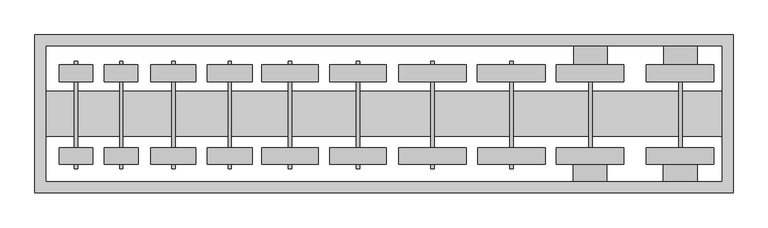
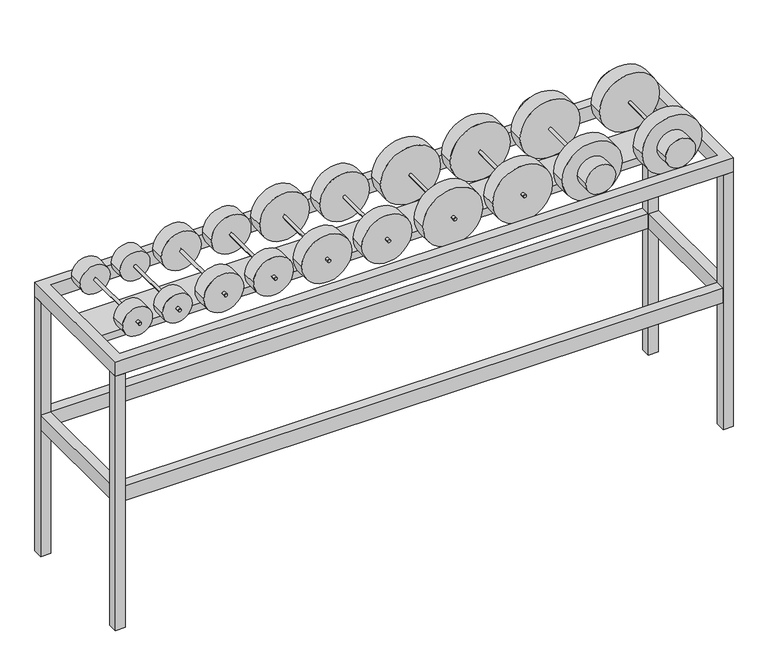
"""IFC4 building model written with IfcOpenShell, lengths in millimetres: proxy geometry."""

from ifc_helpers import new_model, si_unit, point, frame, frame_2d, origin, origin_with_axes, place, context, project, spatial, polyline, circle_curve, trimmed, segment, composite_curve, outline, extrude, source, transform, mapped, element, save


def specialty_equipment_60971a7b(model_context):
    return source(origin(), model_context, "Body", "SweptSolid", [
        extrude(outline(polyline([(-1032.0763254, -159.6107484), (-1032.0763254, 551.5892516), (2117.5236746, 551.5892516), (2117.5236746, -159.6107484), (-1032.0763254, -159.6107484)]), holes=[polyline([(-981.2763254, -108.8107484), (2066.7236746, -108.8107484), (2066.7236746, 500.7892516), (-981.2763254, 500.7892516), (-981.2763254, -108.8107484)])]), origin_with_axes(), (0.0, 0.0, 1.0), 76.2),
        extrude(outline(polyline([(-981.2763254, 500.7892516), (-1032.0763254, 500.7892516), (-1032.0763254, 551.5892516), (-981.2763254, 551.5892516), (-981.2763254, 500.7892516)])), frame((0.0, 0.0, -1371.6), z_axis=(0.0, 0.0, 1.0), x_axis=(1.0, 0.0, 0.0)), (0.0, 0.0, 1.0), 1371.6),
        extrude(outline(polyline([(-981.2763254, -159.6107484), (-1032.0763254, -159.6107484), (-1032.0763254, -108.8107484), (-981.2763254, -108.8107484), (-981.2763254, -159.6107484)])), frame((0.0, 0.0, -1371.6), z_axis=(0.0, 0.0, 1.0), x_axis=(1.0, 0.0, 0.0)), (0.0, 0.0, 1.0), 1371.6),
        extrude(outline(polyline([(2066.7236746, -159.6107484), (2066.7236746, -108.8107484), (2117.5236746, -108.8107484), (2117.5236746, -159.6107484), (2066.7236746, -159.6107484)])), frame((0.0, 0.0, -1371.6), z_axis=(0.0, 0.0, 1.0), x_axis=(1.0, 0.0, 0.0)), (0.0, 0.0, 1.0), 1371.6),
        extrude(outline(polyline([(2066.7236746, 500.7892516), (2066.7236746, 551.5892516), (2117.5236746, 551.5892516), (2117.5236746, 500.7892516), (2066.7236746, 500.7892516)])), frame((0.0, 0.0, -1371.6), z_axis=(0.0, 0.0, 1.0), x_axis=(1.0, 0.0, 0.0)), (0.0, 0.0, 1.0), 1371.6),
        extrude(outline(polyline([(-1032.0763254, -159.6107484), (-1032.0763254, 551.5892516), (2117.5236746, 551.5892516), (2117.5236746, -159.6107484), (-1032.0763254, -159.6107484)]), holes=[polyline([(-981.2763254, -108.8107484), (2066.7236746, -108.8107484), (2066.7236746, 500.7892516), (-981.2763254, 500.7892516), (-981.2763254, -108.8107484)])]), frame((0.0, 0.0, -685.8), z_axis=(0.0, 0.0, 1.0), x_axis=(1.0, 0.0, 0.0)), (0.0, 0.0, 1.0), 76.2),
        extrude(outline(composite_curve([segment(trimmed(circle_curve(frame_2d((154.4606082, -846.3325506)), 76.2), [point((154.4606082, -922.5325506))], [point((154.4606082, -770.1325506))], False, "CARTESIAN"), True, "CONTINUOUS"), segment(trimmed(circle_curve(frame_2d((154.4606082, -846.3325506)), 76.2), [point((154.4606082, -770.1325506))], [point((154.4606082, -922.5325506))], False, "CARTESIAN"), True, "CONTINUOUS")], self_intersect=False)), frame((0.0, -32.5823092, 0.0), z_axis=(0.0, 1.0, 0.0), x_axis=(0.0, 0.0, 1.0)), (0.0, 0.0, 1.0), 76.2),
        extrude(outline(polyline([(-981.2763254, 94.3892516), (-981.2763254, 297.5892516), (2066.7236746, 297.5892516), (2066.7236746, 94.3892516), (-981.2763254, 94.3892516)])), origin_with_axes(), (0.0, 0.0, 1.0), 38.1),
        extrude(outline(composite_curve([segment(trimmed(circle_curve(frame_2d((154.4606082, -846.6284427)), 76.2), [point((154.4606082, -922.8284427))], [point((154.4606082, -770.4284427))], False, "CARTESIAN"), True, "CONTINUOUS"), segment(trimmed(circle_curve(frame_2d((154.4606082, -846.6284427)), 76.2), [point((154.4606082, -770.4284427))], [point((154.4606082, -922.8284427))], False, "CARTESIAN"), True, "CONTINUOUS")], self_intersect=False)), frame((0.0, 341.3226899, 0.0), z_axis=(0.0, 1.0, 0.0), x_axis=(0.0, 0.0, 1.0)), (0.0, 0.0, 1.0), 76.2),
        extrude(outline(composite_curve([segment(trimmed(circle_curve(frame_2d((154.4606082, -845.747476)), 7.8489452), [point((154.4606082, -837.8985309))], [point((154.4606082, -853.5964212))], False, "CARTESIAN"), True, "CONTINUOUS"), segment(trimmed(circle_curve(frame_2d((154.4606082, -845.747476)), 7.8489452), [point((154.4606082, -853.5964212))], [point((154.4606082, -837.8985309))], False, "CARTESIAN"), True, "CONTINUOUS")], self_intersect=False)), frame((0.0, -53.073715, 0.0), z_axis=(0.0, 1.0, 0.0), x_axis=(0.0, 0.0, 1.0)), (0.0, 0.0, 1.0), 485.4827264),
        extrude(outline(composite_curve([segment(trimmed(circle_curve(frame_2d((154.4606082, -643.1325506)), 76.2), [point((154.4606082, -719.3325506))], [point((154.4606082, -566.9325506))], False, "CARTESIAN"), True, "CONTINUOUS"), segment(trimmed(circle_curve(frame_2d((154.4606082, -643.1325506)), 76.2), [point((154.4606082, -566.9325506))], [point((154.4606082, -719.3325506))], False, "CARTESIAN"), True, "CONTINUOUS")], self_intersect=False)), frame((0.0, -32.5823092, 0.0), z_axis=(0.0, 1.0, 0.0), x_axis=(0.0, 0.0, 1.0)), (0.0, 0.0, 1.0), 76.2),
        extrude(outline(composite_curve([segment(trimmed(circle_curve(frame_2d((154.4606082, -643.4284427)), 76.2), [point((154.4606082, -719.6284427))], [point((154.4606082, -567.2284427))], False, "CARTESIAN"), True, "CONTINUOUS"), segment(trimmed(circle_curve(frame_2d((154.4606082, -643.4284427)), 76.2), [point((154.4606082, -567.2284427))], [point((154.4606082, -719.6284427))], False, "CARTESIAN"), True, "CONTINUOUS")], self_intersect=False)), frame((0.0, 341.3226899, 0.0), z_axis=(0.0, 1.0, 0.0), x_axis=(0.0, 0.0, 1.0)), (0.0, 0.0, 1.0), 76.2),
        extrude(outline(composite_curve([segment(trimmed(circle_curve(frame_2d((154.4606082, -642.547476)), 7.8489452), [point((154.4606082, -634.6985309))], [point((154.4606082, -650.3964212))], False, "CARTESIAN"), True, "CONTINUOUS"), segment(trimmed(circle_curve(frame_2d((154.4606082, -642.547476)), 7.8489452), [point((154.4606082, -650.3964212))], [point((154.4606082, -634.6985309))], False, "CARTESIAN"), True, "CONTINUOUS")], self_intersect=False)), frame((0.0, -53.073715, 0.0), z_axis=(0.0, 1.0, 0.0), x_axis=(0.0, 0.0, 1.0)), (0.0, 0.0, 1.0), 485.4827264),
        extrude(outline(composite_curve([segment(trimmed(circle_curve(frame_2d((154.4606082, 1116.9227651)), 152.4), [point((154.4606082, 1269.3227651))], [point((154.4606082, 964.5227651))], False, "CARTESIAN"), True, "CONTINUOUS"), segment(trimmed(circle_curve(frame_2d((154.4606082, 1116.9227651)), 152.4), [point((154.4606082, 964.5227651))], [point((154.4606082, 1269.3227651))], False, "CARTESIAN"), True, "CONTINUOUS")], self_intersect=False)), frame((0.0, -32.5823092, 0.0), z_axis=(0.0, 1.0, 0.0), x_axis=(0.0, 0.0, 1.0)), (0.0, 0.0, 1.0), 76.2),
        extrude(outline(composite_curve([segment(trimmed(circle_curve(frame_2d((154.4606082, 1116.9227651)), 7.8489452), [point((154.4606082, 1124.7717102))], [point((154.4606082, 1109.0738199))], False, "CARTESIAN"), True, "CONTINUOUS"), segment(trimmed(circle_curve(frame_2d((154.4606082, 1116.9227651)), 7.8489452), [point((154.4606082, 1109.0738199))], [point((154.4606082, 1124.7717102))], False, "CARTESIAN"), True, "CONTINUOUS")], self_intersect=False)), frame((0.0, -53.073715, 0.0), z_axis=(0.0, 1.0, 0.0), x_axis=(0.0, 0.0, 1.0)), (0.0, 0.0, 1.0), 485.4827264),
        extrude(outline(composite_curve([segment(trimmed(circle_curve(frame_2d((154.4606082, 1116.7428206)), 152.4), [point((154.4606082, 1269.1428206))], [point((154.4606082, 964.3428206))], False, "CARTESIAN"), True, "CONTINUOUS"), segment(trimmed(circle_curve(frame_2d((154.4606082, 1116.7428206)), 152.4), [point((154.4606082, 964.3428206))], [point((154.4606082, 1269.1428206))], False, "CARTESIAN"), True, "CONTINUOUS")], self_intersect=False)), frame((0.0, 341.3226899, 0.0), z_axis=(0.0, 1.0, 0.0), x_axis=(0.0, 0.0, 1.0)), (0.0, 0.0, 1.0), 76.2),
        extrude(outline(composite_curve([segment(trimmed(circle_curve(frame_2d((154.4606082, 761.3227651)), 152.4), [point((154.4606082, 913.7227651))], [point((154.4606082, 608.9227651))], False, "CARTESIAN"), True, "CONTINUOUS"), segment(trimmed(circle_curve(frame_2d((154.4606082, 761.3227651)), 152.4), [point((154.4606082, 608.9227651))], [point((154.4606082, 913.7227651))], False, "CARTESIAN"), True, "CONTINUOUS")], self_intersect=False)), frame((0.0, -32.5823092, 0.0), z_axis=(0.0, 1.0, 0.0), x_axis=(0.0, 0.0, 1.0)), (0.0, 0.0, 1.0), 76.2),
        extrude(outline(composite_curve([segment(trimmed(circle_curve(frame_2d((154.4606082, 761.3227651)), 7.8489452), [point((154.4606082, 769.1717102))], [point((154.4606082, 753.4738199))], False, "CARTESIAN"), True, "CONTINUOUS"), segment(trimmed(circle_curve(frame_2d((154.4606082, 761.3227651)), 7.8489452), [point((154.4606082, 753.4738199))], [point((154.4606082, 769.1717102))], False, "CARTESIAN"), True, "CONTINUOUS")], self_intersect=False)), frame((0.0, -53.073715, 0.0), z_axis=(0.0, 1.0, 0.0), x_axis=(0.0, 0.0, 1.0)), (0.0, 0.0, 1.0), 485.4827264),
        extrude(outline(composite_curve([segment(trimmed(circle_curve(frame_2d((154.4606082, 761.1428206)), 152.4), [point((154.4606082, 913.5428206))], [point((154.4606082, 608.7428206))], False, "CARTESIAN"), True, "CONTINUOUS"), segment(trimmed(circle_curve(frame_2d((154.4606082, 761.1428206)), 152.4), [point((154.4606082, 608.7428206))], [point((154.4606082, 913.5428206))], False, "CARTESIAN"), True, "CONTINUOUS")], self_intersect=False)), frame((0.0, 341.3226899, 0.0), z_axis=(0.0, 1.0, 0.0), x_axis=(0.0, 0.0, 1.0)), (0.0, 0.0, 1.0), 76.2),
        extrude(outline(composite_curve([segment(trimmed(circle_curve(frame_2d((154.4606082, -407.0772349)), 101.6), [point((154.4606082, -305.4772349))], [point((154.4606082, -508.6772349))], False, "CARTESIAN"), True, "CONTINUOUS"), segment(trimmed(circle_curve(frame_2d((154.4606082, -407.0772349)), 101.6), [point((154.4606082, -508.6772349))], [point((154.4606082, -305.4772349))], False, "CARTESIAN"), True, "CONTINUOUS")], self_intersect=False)), frame((0.0, -32.5823092, 0.0), z_axis=(0.0, 1.0, 0.0), x_axis=(0.0, 0.0, 1.0)), (0.0, 0.0, 1.0), 76.2),
        extrude(outline(composite_curve([segment(trimmed(circle_curve(frame_2d((154.4606082, -407.0772349)), 7.8489452), [point((154.4606082, -399.2282898))], [point((154.4606082, -414.9261801))], False, "CARTESIAN"), True, "CONTINUOUS"), segment(trimmed(circle_curve(frame_2d((154.4606082, -407.0772349)), 7.8489452), [point((154.4606082, -414.9261801))], [point((154.4606082, -399.2282898))], False, "CARTESIAN"), True, "CONTINUOUS")], self_intersect=False)), frame((0.0, -53.073715, 0.0), z_axis=(0.0, 1.0, 0.0), x_axis=(0.0, 0.0, 1.0)), (0.0, 0.0, 1.0), 485.4827264),
        extrude(outline(composite_curve([segment(trimmed(circle_curve(frame_2d((154.4606082, -407.2571794)), 101.6), [point((154.4606082, -305.6571794))], [point((154.4606082, -508.8571794))], False, "CARTESIAN"), True, "CONTINUOUS"), segment(trimmed(circle_curve(frame_2d((154.4606082, -407.2571794)), 101.6), [point((154.4606082, -508.8571794))], [point((154.4606082, -305.6571794))], False, "CARTESIAN"), True, "CONTINUOUS")], self_intersect=False)), frame((0.0, 341.3226899, 0.0), z_axis=(0.0, 1.0, 0.0), x_axis=(0.0, 0.0, 1.0)), (0.0, 0.0, 1.0), 76.2),
        extrude(outline(composite_curve([segment(trimmed(circle_curve(frame_2d((154.4606082, -153.0772349)), 101.6), [point((154.4606082, -51.4772349))], [point((154.4606082, -254.6772349))], False, "CARTESIAN"), True, "CONTINUOUS"), segment(trimmed(circle_curve(frame_2d((154.4606082, -153.0772349)), 101.6), [point((154.4606082, -254.6772349))], [point((154.4606082, -51.4772349))], False, "CARTESIAN"), True, "CONTINUOUS")], self_intersect=False)), frame((0.0, -32.5823092, 0.0), z_axis=(0.0, 1.0, 0.0), x_axis=(0.0, 0.0, 1.0)), (0.0, 0.0, 1.0), 76.2),
        extrude(outline(composite_curve([segment(trimmed(circle_curve(frame_2d((154.4606082, -153.0772349)), 7.8489452), [point((154.4606082, -145.2282898))], [point((154.4606082, -160.9261801))], False, "CARTESIAN"), True, "CONTINUOUS"), segment(trimmed(circle_curve(frame_2d((154.4606082, -153.0772349)), 7.8489452), [point((154.4606082, -160.9261801))], [point((154.4606082, -145.2282898))], False, "CARTESIAN"), True, "CONTINUOUS")], self_intersect=False)), frame((0.0, -53.073715, 0.0), z_axis=(0.0, 1.0, 0.0), x_axis=(0.0, 0.0, 1.0)), (0.0, 0.0, 1.0), 485.4827264),
        extrude(outline(composite_curve([segment(trimmed(circle_curve(frame_2d((154.4606082, -153.2571794)), 101.6), [point((154.4606082, -51.6571794))], [point((154.4606082, -254.8571794))], False, "CARTESIAN"), True, "CONTINUOUS"), segment(trimmed(circle_curve(frame_2d((154.4606082, -153.2571794)), 101.6), [point((154.4606082, -254.8571794))], [point((154.4606082, -51.6571794))], False, "CARTESIAN"), True, "CONTINUOUS")], self_intersect=False)), frame((0.0, 341.3226899, 0.0), z_axis=(0.0, 1.0, 0.0), x_axis=(0.0, 0.0, 1.0)), (0.0, 0.0, 1.0), 76.2),
        extrude(outline(composite_curve([segment(trimmed(circle_curve(frame_2d((154.4606082, 119.2581533)), 127.0), [point((154.4606082, 246.2581533))], [point((154.4606082, -7.7418467))], False, "CARTESIAN"), True, "CONTINUOUS"), segment(trimmed(circle_curve(frame_2d((154.4606082, 119.2581533)), 127.0), [point((154.4606082, -7.7418467))], [point((154.4606082, 246.2581533))], False, "CARTESIAN"), True, "CONTINUOUS")], self_intersect=False)), frame((0.0, -32.5823092, 0.0), z_axis=(0.0, 1.0, 0.0), x_axis=(0.0, 0.0, 1.0)), (0.0, 0.0, 1.0), 76.2),
        extrude(outline(composite_curve([segment(trimmed(circle_curve(frame_2d((154.4606082, 119.2581533)), 7.8489452), [point((154.4606082, 127.1070985))], [point((154.4606082, 111.4092081))], False, "CARTESIAN"), True, "CONTINUOUS"), segment(trimmed(circle_curve(frame_2d((154.4606082, 119.2581533)), 7.8489452), [point((154.4606082, 111.4092081))], [point((154.4606082, 127.1070985))], False, "CARTESIAN"), True, "CONTINUOUS")], self_intersect=False)), frame((0.0, -53.073715, 0.0), z_axis=(0.0, 1.0, 0.0), x_axis=(0.0, 0.0, 1.0)), (0.0, 0.0, 1.0), 485.4827264),
        extrude(outline(composite_curve([segment(trimmed(circle_curve(frame_2d((154.4606082, 119.0782088)), 127.0), [point((154.4606082, 246.0782088))], [point((154.4606082, -7.9217912))], False, "CARTESIAN"), True, "CONTINUOUS"), segment(trimmed(circle_curve(frame_2d((154.4606082, 119.0782088)), 127.0), [point((154.4606082, -7.9217912))], [point((154.4606082, 246.0782088))], False, "CARTESIAN"), True, "CONTINUOUS")], self_intersect=False)), frame((0.0, 341.3226899, 0.0), z_axis=(0.0, 1.0, 0.0), x_axis=(0.0, 0.0, 1.0)), (0.0, 0.0, 1.0), 76.2),
        extrude(outline(composite_curve([segment(trimmed(circle_curve(frame_2d((154.4606082, 425.128062)), 127.0), [point((154.4606082, 552.128062))], [point((154.4606082, 298.128062))], False, "CARTESIAN"), True, "CONTINUOUS"), segment(trimmed(circle_curve(frame_2d((154.4606082, 425.128062)), 127.0), [point((154.4606082, 298.128062))], [point((154.4606082, 552.128062))], False, "CARTESIAN"), True, "CONTINUOUS")], self_intersect=False)), frame((0.0, -32.5823092, 0.0), z_axis=(0.0, 1.0, 0.0), x_axis=(0.0, 0.0, 1.0)), (0.0, 0.0, 1.0), 76.2),
        extrude(outline(composite_curve([segment(trimmed(circle_curve(frame_2d((154.4606082, 425.128062)), 7.8489452), [point((154.4606082, 432.9770072))], [point((154.4606082, 417.2791168))], False, "CARTESIAN"), True, "CONTINUOUS"), segment(trimmed(circle_curve(frame_2d((154.4606082, 425.128062)), 7.8489452), [point((154.4606082, 417.2791168))], [point((154.4606082, 432.9770072))], False, "CARTESIAN"), True, "CONTINUOUS")], self_intersect=False)), frame((0.0, -53.073715, 0.0), z_axis=(0.0, 1.0, 0.0), x_axis=(0.0, 0.0, 1.0)), (0.0, 0.0, 1.0), 485.4827264),
        extrude(outline(composite_curve([segment(trimmed(circle_curve(frame_2d((154.4606082, 424.9481175)), 127.0), [point((154.4606082, 551.9481175))], [point((154.4606082, 297.9481175))], False, "CARTESIAN"), True, "CONTINUOUS"), segment(trimmed(circle_curve(frame_2d((154.4606082, 424.9481175)), 127.0), [point((154.4606082, 297.9481175))], [point((154.4606082, 551.9481175))], False, "CARTESIAN"), True, "CONTINUOUS")], self_intersect=False)), frame((0.0, 341.3226899, 0.0), z_axis=(0.0, 1.0, 0.0), x_axis=(0.0, 0.0, 1.0)), (0.0, 0.0, 1.0), 76.2),
        extrude(outline(composite_curve([segment(trimmed(circle_curve(frame_2d((154.4606082, 1878.6053565)), 76.2), [point((154.4606082, 1802.4053565))], [point((154.4606082, 1954.8053565))], False, "CARTESIAN"), True, "CONTINUOUS"), segment(trimmed(circle_curve(frame_2d((154.4606082, 1878.6053565)), 76.2), [point((154.4606082, 1954.8053565))], [point((154.4606082, 1802.4053565))], False, "CARTESIAN"), True, "CONTINUOUS")], self_intersect=False)), frame((0.0, -108.7823092, 0.0), z_axis=(0.0, 1.0, 0.0), x_axis=(0.0, 0.0, 1.0)), (0.0, 0.0, 1.0), 76.2),
        extrude(outline(composite_curve([segment(trimmed(circle_curve(frame_2d((154.4606082, 1880.3392515)), 76.2), [point((154.4606082, 1804.1392515))], [point((154.4606082, 1956.5392515))], False, "CARTESIAN"), True, "CONTINUOUS"), segment(trimmed(circle_curve(frame_2d((154.4606082, 1880.3392515)), 76.2), [point((154.4606082, 1956.5392515))], [point((154.4606082, 1804.1392515))], False, "CARTESIAN"), True, "CONTINUOUS")], self_intersect=False)), frame((0.0, 417.5226899, 0.0), z_axis=(0.0, 1.0, 0.0), x_axis=(0.0, 0.0, 1.0)), (0.0, 0.0, 1.0), 83.2665617),
        extrude(outline(composite_curve([segment(trimmed(circle_curve(frame_2d((154.4606082, 1878.7428206)), 152.4), [point((154.4606082, 2031.1428206))], [point((154.4606082, 1726.3428206))], False, "CARTESIAN"), True, "CONTINUOUS"), segment(trimmed(circle_curve(frame_2d((154.4606082, 1878.7428206)), 152.4), [point((154.4606082, 1726.3428206))], [point((154.4606082, 2031.1428206))], False, "CARTESIAN"), True, "CONTINUOUS")], self_intersect=False)), frame((0.0, 341.3226899, 0.0), z_axis=(0.0, 1.0, 0.0), x_axis=(0.0, 0.0, 1.0)), (0.0, 0.0, 1.0), 76.2),
        extrude(outline(composite_curve([segment(trimmed(circle_curve(frame_2d((154.4606082, 1878.9227651)), 152.4), [point((154.4606082, 2031.3227651))], [point((154.4606082, 1726.5227651))], False, "CARTESIAN"), True, "CONTINUOUS"), segment(trimmed(circle_curve(frame_2d((154.4606082, 1878.9227651)), 152.4), [point((154.4606082, 1726.5227651))], [point((154.4606082, 2031.3227651))], False, "CARTESIAN"), True, "CONTINUOUS")], self_intersect=False)), frame((0.0, -32.5823092, 0.0), z_axis=(0.0, 1.0, 0.0), x_axis=(0.0, 0.0, 1.0)), (0.0, 0.0, 1.0), 76.2),
        extrude(outline(composite_curve([segment(trimmed(circle_curve(frame_2d((154.4606082, 1880.0953579)), 7.8489452), [point((154.4606082, 1887.9443031))], [point((154.4606082, 1872.2464127))], False, "CARTESIAN"), True, "CONTINUOUS"), segment(trimmed(circle_curve(frame_2d((154.4606082, 1880.0953579)), 7.8489452), [point((154.4606082, 1872.2464127))], [point((154.4606082, 1887.9443031))], False, "CARTESIAN"), True, "CONTINUOUS")], self_intersect=False)), frame((0.0, -89.1618249, 0.0), z_axis=(0.0, 1.0, 0.0), x_axis=(0.0, 0.0, 1.0)), (0.0, 0.0, 1.0), 555.3477574),
        extrude(outline(composite_curve([segment(trimmed(circle_curve(frame_2d((154.4606082, 1472.2053565)), 76.2), [point((154.4606082, 1396.0053565))], [point((154.4606082, 1548.4053565))], False, "CARTESIAN"), True, "CONTINUOUS"), segment(trimmed(circle_curve(frame_2d((154.4606082, 1472.2053565)), 76.2), [point((154.4606082, 1548.4053565))], [point((154.4606082, 1396.0053565))], False, "CARTESIAN"), True, "CONTINUOUS")], self_intersect=False)), frame((0.0, -108.7823092, 0.0), z_axis=(0.0, 1.0, 0.0), x_axis=(0.0, 0.0, 1.0)), (0.0, 0.0, 1.0), 76.2),
        extrude(outline(composite_curve([segment(trimmed(circle_curve(frame_2d((154.4606082, 1473.9392515)), 76.2), [point((154.4606082, 1397.7392515))], [point((154.4606082, 1550.1392515))], False, "CARTESIAN"), True, "CONTINUOUS"), segment(trimmed(circle_curve(frame_2d((154.4606082, 1473.9392515)), 76.2), [point((154.4606082, 1550.1392515))], [point((154.4606082, 1397.7392515))], False, "CARTESIAN"), True, "CONTINUOUS")], self_intersect=False)), frame((0.0, 417.5226899, 0.0), z_axis=(0.0, 1.0, 0.0), x_axis=(0.0, 0.0, 1.0)), (0.0, 0.0, 1.0), 83.2665617),
        extrude(outline(composite_curve([segment(trimmed(circle_curve(frame_2d((154.4606082, 1472.3428206)), 152.4), [point((154.4606082, 1624.7428206))], [point((154.4606082, 1319.9428206))], False, "CARTESIAN"), True, "CONTINUOUS"), segment(trimmed(circle_curve(frame_2d((154.4606082, 1472.3428206)), 152.4), [point((154.4606082, 1319.9428206))], [point((154.4606082, 1624.7428206))], False, "CARTESIAN"), True, "CONTINUOUS")], self_intersect=False)), frame((0.0, 341.3226899, 0.0), z_axis=(0.0, 1.0, 0.0), x_axis=(0.0, 0.0, 1.0)), (0.0, 0.0, 1.0), 76.2),
        extrude(outline(composite_curve([segment(trimmed(circle_curve(frame_2d((154.4606082, 1472.5227651)), 152.4), [point((154.4606082, 1624.9227651))], [point((154.4606082, 1320.1227651))], False, "CARTESIAN"), True, "CONTINUOUS"), segment(trimmed(circle_curve(frame_2d((154.4606082, 1472.5227651)), 152.4), [point((154.4606082, 1320.1227651))], [point((154.4606082, 1624.9227651))], False, "CARTESIAN"), True, "CONTINUOUS")], self_intersect=False)), frame((0.0, -32.5823092, 0.0), z_axis=(0.0, 1.0, 0.0), x_axis=(0.0, 0.0, 1.0)), (0.0, 0.0, 1.0), 76.2),
        extrude(outline(composite_curve([segment(trimmed(circle_curve(frame_2d((154.4606082, 1473.6953579)), 7.8489452), [point((154.4606082, 1481.5443031))], [point((154.4606082, 1465.8464127))], False, "CARTESIAN"), True, "CONTINUOUS"), segment(trimmed(circle_curve(frame_2d((154.4606082, 1473.6953579)), 7.8489452), [point((154.4606082, 1465.8464127))], [point((154.4606082, 1481.5443031))], False, "CARTESIAN"), True, "CONTINUOUS")], self_intersect=False)), frame((0.0, -89.1618249, 0.0), z_axis=(0.0, 1.0, 0.0), x_axis=(0.0, 0.0, 1.0)), (0.0, 0.0, 1.0), 555.3477574),
    ])


if __name__ == "__main__":
    model = new_model("IFC4")
    model_context = context("Model", 3, world=origin())
    ifc_project = project(units=[si_unit("LENGTHUNIT", "METRE", prefix="MILLI")], contexts=[model_context])
    site = spatial("IfcSite", under=ifc_project)
    building = spatial("IfcBuilding", under=site)
    placement = place(None, origin())
    specialty_equipment_shape = specialty_equipment_60971a7b(model_context)
    element("IfcBuildingElementProxy", 1, Name="Specialty Equipment", at=placement, inside=building, context=model_context, shape_type="MappedRepresentation", body=[
        mapped(specialty_equipment_shape, transform((0.0, 0.0, 0.0), x_axis=(1.0, 0.0, 0.0), y_axis=(0.0, 1.0, 0.0), z_axis=(0.0, 0.0, 1.0))),
    ])
    save(model, "model.ifc")

# Revit data of these elements
# Type
#   Default Elevation = 0
